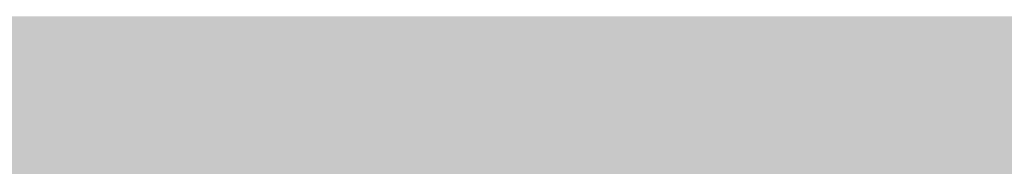
# Model space of a CAD drawing. Units: feet. Extents: x 3168 to 4724, y 827 to 1477.
# Tile 20 of 256: x 3257.497 to 3261.901, y 1098.344 to 1099.001. Entities that reach past the tile are written whole.
import ezdxf

# ---------------------------------------------------------------- set-up
doc = ezdxf.new("R2010")
doc.units = ezdxf.units.FT
doc.layers.add('A-ELEV', color=7, linetype='Continuous', lineweight=35)
doc.layers.add('A-ELEV-PATT', color=8, linetype='Continuous', lineweight=13)

msp = doc.modelspace()

# ---------------------------------------------------------------- hatches: boundary and pattern name
at = {"layer": 'A-ELEV-PATT'}
h = msp.add_hatch(color=256, dxfattribs=at)
h.dxf.hatch_style = 1
edge = h.paths.add_edge_path()
edge.add_ellipse((3552.9058, 979.2201), major_axis=(36.7449, 0), ratio=0.4848485, start_angle=0, end_angle=360)
edge = h.paths.add_edge_path()
edge.add_ellipse((3559.8916, 929.2523), major_axis=(36.7449, 0), ratio=0.4848485, start_angle=0, end_angle=360)
edge = h.paths.add_edge_path()
edge.add_line((3299.3168, 1198.6061), (3479.9167, 1198.6061))
edge.add_line((3479.9167, 1198.6061), (3479.9167, 1209.8686))
edge.add_spline(control_points=[(3479.9167, 1209.8686), (3464.3012, 1209.8686), (3448.6856, 1209.8686), (3410.9491, 1209.8686), (3388.8282, 1209.8686), (3355.6469, 1209.8686), (3344.5864, 1209.8686), (3327.9957, 1209.8686), (3322.4655, 1209.8686), (3314.1702, 1209.8686), (3311.4051, 1209.8686), (3307.2574, 1209.8686), (3305.8748, 1209.8686), (3303.801, 1209.8686), (3303.1097, 1209.8686), (3302.0728, 1209.8686), (3301.7272, 1209.8686), (3301.2087, 1209.8686), (3301.0359, 1209.8686), (3300.7767, 1209.8686), (3300.6903, 1209.8686), (3300.5606, 1209.8686), (3300.5174, 1209.8686), (3300.4526, 1209.8686), (3300.431, 1209.8686), (3300.3986, 1209.8686), (3300.3878, 1209.8686), (3300.3662, 1209.8686), (3300.3457, 1209.8686), (3300.3455, 1209.8686), (3300.3455, 1209.8686), (3300.3433, 1209.8686), (3300.3411, 1209.8686), (3300.3379, 1209.8686), (3300.3368, 1209.8686), (3300.3339, 1209.8686), (3300.3321, 1209.8686), (3300.3255, 1209.8686), (3300.3207, 1209.8686), (3300.3109, 1209.8686), (3300.306, 1209.8686), (3300.2905, 1209.8686), (3300.28, 1209.8686), (3300.2324, 1209.8688), (3300.1953, 1209.869), (3299.9511, 1209.8706), (3299.7448, 1209.8743), (3299.4368, 1209.8833), (3299.3344, 1209.8868), (3299.1811, 1209.8929), (3299.13, 1209.8951), (3298.6522, 1209.9168), (3298.2295, 1209.9457), (3297.6016, 1210.0024), (3297.3934, 1210.0235), (3297.0827, 1210.0583), (3296.9793, 1210.0705), (3296.293, 1210.1549), (3295.7181, 1210.2434), (3294.8687, 1210.3989), (3294.5877, 1210.4545), (3294.1693, 1210.5433), (3294.0304, 1210.5739), (3291.7071, 1211.1012), (3289.6536, 1211.8134), (3285.7763, 1213.564), (3283.9514, 1214.6035), (3280.5122, 1216.9801), (3278.8972, 1218.3176), (3276.3799, 1220.8295), (3275.416, 1221.9177), (3274.0393, 1223.7077), (3273.581, 1224.3495), (3273.1432, 1225.0163)], knot_values=[39.119033, 39.119033, 39.119033, 39.119033, 39.286353, 39.286353, 39.523379, 39.523379, 39.641892, 39.641892, 39.701148, 39.701148, 39.730777, 39.730777, 39.745591, 39.745591, 39.752998, 39.752998, 39.756701, 39.756701, 39.758553, 39.758553, 39.759479, 39.759479, 39.759942, 39.759942, 39.760173, 39.760173, 39.760289, 39.760289, 39.760405, 39.760405, 39.760463, 39.760463, 39.763389, 39.763389, 39.764851, 39.764851, 39.767304, 39.767304, 39.773825, 39.773825, 39.78057, 39.78057, 39.79477, 39.79477, 39.845194, 39.845194, 40.126715, 40.126715, 40.267476, 40.267476, 40.337856, 40.337856, 40.927023, 40.927023, 41.221606, 41.221606, 41.368898, 41.368898, 42.202622, 42.202622, 42.619485, 42.619485, 42.827916, 42.827916, 46.118323, 46.118323, 49.408731, 49.408731, 52.699139, 52.699139, 54.927489, 54.927489, 56.104228, 56.104228, 56.104228, 56.104228], weights=[1, 1, 1, 1, 1, 1, 1, 1, 1, 1, 1, 1, 1, 1, 1, 1, 1, 1, 1, 1, 1, 1, 1, 1, 1, 1, 1, 1, 1, 1, 1, 1, 1, 1, 1, 1, 1, 1, 1, 1, 1, 1, 1, 1, 1, 1, 1, 1, 1, 1, 1, 1, 1, 1, 1, 1, 1, 1, 1, 1, 1, 1, 1, 1, 1, 1, 1, 1, 1, 1, 1, 1, 1, 1], degree=3, periodic=0)
edge.add_line((3273.1432, 1225.0163), (3273.1432, 1099.0163))
edge.add_line((3273.1432, 1099.0163), (3299.3168, 1099.0163))
edge.add_line((3299.3168, 1099.0163), (3299.3168, 1198.6061))
edge = h.paths.add_edge_path()
edge.add_line((3304.7584, 1324.1581), (3479.9167, 1324.1581))
edge.add_line((3479.9167, 1324.1581), (3479.9167, 1335.7146))
edge.add_line((3479.9167, 1335.7146), (3269.1616, 1335.7146))
edge.add_spline(control_points=[(3269.1616, 1335.7146), (3264.0242, 1335.7146), (3258.3641, 1328.9582), (3259.2643, 1323.9003)], knot_values=[0, 0, 0, 0, 15.412191, 15.412191, 15.412191, 15.412191], degree=3, periodic=0)
edge.add_line((3259.2643, 1323.9003), (3265.5168, 1288.7691))
edge.add_line((3265.5168, 1288.7691), (3275.2651, 1261.5456))
edge.add_line((3275.2651, 1261.5456), (3304.7584, 1261.5456))
edge.add_line((3304.7584, 1261.5456), (3304.7584, 1324.1581))
h = msp.add_hatch(color=256, dxfattribs=at)
h.dxf.hatch_style = 1
h.paths.add_polyline_path([(3384.5252, 1099.0163), (3335.0292, 1099.0163), (3299.3168, 1099.0163), (3273.1432, 1099.0163), (3217.5654, 1099.0163), (3168.0693, 827.1163), (3335.0292, 827.1163)])

# ---------------------------------------------------------------- linework, layer by layer
at = {"layer": 'A-ELEV'}
msp.add_open_spline([(3808.5202, 1099.0163), (3808.5202, 1141.4132), (3808.5202, 1183.8102), (3808.5202, 1226.6353), (3808.5202, 1227.0636), (3808.5202, 1227.4918), (3811.4919, 1248.9947), (3814.4635, 1270.4975), (3817.4652, 1292.2176), (3817.4952, 1292.4348), (3817.5253, 1292.652), (3817.5728, 1310.1067), (3817.6203, 1327.5615), (3817.6679, 1345.0163), (3817.6679, 1345.458), (3817.6679, 1345.8996), (3817.6679, 1346.456), (3817.6679, 1346.5708), (3817.6679, 1346.7529), (3817.6679, 1346.8201), (3817.6679, 1346.9349), (3817.6679, 1346.9823), (3817.6679, 1347.0386), (3817.6679, 1347.0474), (3817.6679, 1347.0737), (3817.6679, 1347.0593), (3817.6679, 1347.0615), (3817.6679, 1347.0627), (3817.6679, 1347.066), (3817.6679, 1347.0683), (3817.6679, 1347.075), (3817.6679, 1347.0795), (3817.6678, 1347.0929), (3817.6678, 1347.1019), (3817.6678, 1347.1288), (3817.6677, 1347.1467), (3817.6674, 1347.2004), (3817.6672, 1347.2362), (3817.6661, 1347.3434), (3817.665, 1347.4147), (3817.6608, 1347.6281), (3817.6566, 1347.7697), (3817.64, 1348.1925), (3817.6235, 1348.4716), (3817.5591, 1349.3001), (3817.4961, 1349.8406), (3817.2554, 1351.4242), (3817.0263, 1352.4288), (3816.3069, 1354.8889), (3815.7437, 1356.2687), (3814.464, 1358.8192), (3813.7464, 1359.991), (3812.1958, 1362.1723), (3811.3622, 1363.1821), (3809.5888, 1365.069), (3808.6488, 1365.9461), (3806.6543, 1367.5796), (3805.5997, 1368.3362), (3803.3529, 1369.7223), (3802.1605, 1370.3524), (3799.6008, 1371.4536), (3798.2327, 1371.9255), (3795.2801, 1372.6346), (3793.6931, 1372.8721), (3791.8694, 1372.9265), (3791.7409, 1372.9292), (3791.3534, 1372.9341), (3791.0927, 1372.9329), (3790.3041, 1372.9151), (3789.7695, 1372.8842), (3789.2092, 1372.8302), (3789.1906, 1372.8284), (3789.1349, 1372.8229), (3789.0977, 1372.8191), (3789.0484, 1372.814), (3789.0364, 1372.8127), (3789.0003, 1372.8089), (3788.9761, 1372.8063), (3788.9494, 1372.8034), (3788.9468, 1372.8031), (3788.9426, 1372.8027), (3788.941, 1372.8025), (3788.9386, 1372.8022), (3788.9378, 1372.8021), (3788.9354, 1372.8019), (3788.8675, 1372.7944), (3788.7569, 1372.7822), (3788.7015, 1372.7761), (3788.5355, 1372.7579), (3788.4249, 1372.7457), (3788.0929, 1372.7092), (3787.8715, 1372.6848), (3787.2075, 1372.6118), (3786.7648, 1372.5631), (3785.4368, 1372.417), (3784.5515, 1372.3196), (3781.8954, 1372.0274), (3780.1247, 1371.8327), (3774.8126, 1371.2483), (3771.2713, 1370.8587), (3760.6471, 1369.69), (3753.5643, 1368.9109), (3732.316, 1366.5735), (3718.1504, 1365.0152), (3694.0068, 1362.3593), (3684.0287, 1361.2617), (3674.0506, 1360.1641), (3664.6007, 1360.1641), (3655.1508, 1360.1641), (3626.8011, 1360.1641), (3607.9013, 1360.1641), (3551.2019, 1360.1641), (3513.4023, 1360.1641), (3467.7252, 1360.1641), (3459.8476, 1360.1641), (3436.2149, 1360.1641), (3420.4597, 1360.1641), (3373.1943, 1360.1641), (3341.6839, 1360.1641), (3302.8482, 1360.1641), (3295.5227, 1360.1641), (3286.0383, 1360.1641), (3283.8794, 1360.1641), (3277.4026, 1360.1641), (3273.0848, 1360.1641), (3267.7329, 1360.1641), (3266.6988, 1360.1641), (3263.5965, 1360.1641), (3261.5284, 1360.1641), (3259.2369, 1360.1641), (3259.0137, 1360.1641), (3258.344, 1360.1641), (3257.8975, 1360.1641), (3257.431, 1360.1641), (3257.411, 1360.1641), (3257.3706, 1360.1641), (3257.3755, 1360.1641), (3257.3746, 1360.1641), (3257.3739, 1360.1641), (3257.372, 1360.1641), (3257.3706, 1360.1641), (3257.3667, 1360.1641), (3257.364, 1360.1641), (3257.3561, 1360.1641), (3257.3508, 1360.164), (3257.335, 1360.164), (3257.3244, 1360.164), (3257.2928, 1360.1639), (3257.2717, 1360.1638), (3257.2084, 1360.1634), (3257.1663, 1360.163), (3257.0402, 1360.1614), (3256.9563, 1360.1598), (3256.7055, 1360.1534), (3256.5392, 1360.147), (3256.0436, 1360.1219), (3255.7173, 1360.0971), (3254.7524, 1360.0005), (3254.128, 1359.9065), (3252.1801, 1359.5253), (3250.9416, 1359.144), (3248.6702, 1358.2433), (3247.6357, 1357.7238), (3245.7326, 1356.6035), (3244.8634, 1356.0021), (3243.2531, 1354.7429), (3242.512, 1354.0847), (3240.7511, 1352.3448), (3239.801, 1351.2296), (3238.0878, 1348.8724), (3237.3247, 1347.6304), (3235.9825, 1344.9716), (3235.4022, 1343.5549), (3234.5911, 1340.8155), (3234.3109, 1339.5435), (3233.9765, 1336.8026), (3233.9221, 1335.3309), (3234.1489, 1332.5913), (3234.3495, 1331.3672), (3234.7199, 1329.9994), (3234.7524, 1329.8834), (3234.8536, 1329.5348), (3234.9259, 1329.3017), (3235.0248, 1329.0026), (3235.0469, 1328.9369), (3235.0776, 1328.8472), (3235.0859, 1328.8232), (3235.1109, 1328.7511), (3235.1278, 1328.703), (3235.148, 1328.6462), (3235.1511, 1328.6376), (3235.1561, 1328.6235), (3235.1581, 1328.618), (3235.1602, 1328.612), (3235.1656, 1328.5969), (3235.1801, 1328.5565), (3235.1903, 1328.5281), (3235.2208, 1328.4429), (3235.2411, 1328.3862), (3235.3021, 1328.2159), (3235.3427, 1328.1023), (3235.4647, 1327.7617), (3235.546, 1327.5346), (3235.79, 1326.8534), (3235.9526, 1326.3992), (3236.4405, 1325.0367), (3236.7657, 1324.1284), (3237.7415, 1321.4034), (3238.392, 1319.5868), (3240.3435, 1314.1369), (3241.6445, 1310.5036), (3245.5476, 1299.6037), (3248.1496, 1292.3371), (3255.9557, 1270.5374), (3261.1598, 1256.0042), (3267.3876, 1238.612), (3268.4114, 1235.7529), (3269.5104, 1232.6839), (3269.5856, 1232.4739), (3269.7066, 1232.1359), (3269.7524, 1232.0079), (3269.8273, 1231.7987), (3269.8564, 1231.7176), (3269.9063, 1231.5781), (3269.9272, 1231.5198), (3269.9725, 1231.3934), (3269.9968, 1231.3254), (3270.0265, 1231.2425), (3270.0318, 1231.2277), (3270.0403, 1231.204), (3270.0392, 1231.207), (3270.0394, 1231.2066), (3270.0394, 1231.2064), (3270.0396, 1231.2058), (3270.0398, 1231.2055), (3270.0402, 1231.2043), (3270.0404, 1231.2036), (3270.0413, 1231.2013), (3270.0418, 1231.1998), (3270.0434, 1231.1953), (3270.0445, 1231.1922), (3270.0478, 1231.1832), (3270.0499, 1231.1771), (3270.0564, 1231.159), (3270.0608, 1231.147), (3270.0739, 1231.1108), (3270.0826, 1231.0867), (3270.1089, 1231.0144), (3270.1266, 1230.9663), (3270.1799, 1230.8225), (3270.2159, 1230.7269), (3270.3253, 1230.4415), (3270.4, 1230.2528), (3270.6292, 1229.6914), (3270.7889, 1229.3235), (3271.2865, 1228.2383), (3271.6431, 1227.5398), (3272.7759, 1225.5153), (3273.6142, 1224.2605), (3275.416, 1221.9177), (3276.3799, 1220.8295), (3278.8972, 1218.3176), (3280.5122, 1216.9801), (3283.9514, 1214.6035), (3285.7763, 1213.564), (3289.6536, 1211.8134), (3291.7071, 1211.1012), (3294.0304, 1210.5739), (3294.1693, 1210.5433), (3294.5877, 1210.4545), (3294.8687, 1210.3989), (3295.7181, 1210.2434), (3296.293, 1210.1549), (3296.9793, 1210.0705), (3297.0827, 1210.0583), (3297.3934, 1210.0235), (3297.6016, 1210.0024), (3298.2295, 1209.9457), (3298.6522, 1209.9168), (3299.13, 1209.8951), (3299.1811, 1209.8929), (3299.3344, 1209.8868), (3299.4368, 1209.8833), (3299.7448, 1209.8743), (3299.9511, 1209.8706), (3300.1953, 1209.869), (3300.2324, 1209.8688), (3300.28, 1209.8686), (3300.2905, 1209.8686), (3300.306, 1209.8686), (3300.3109, 1209.8686), (3300.3207, 1209.8686), (3300.3255, 1209.8686), (3300.3321, 1209.8686), (3300.3339, 1209.8686), (3300.3368, 1209.8686), (3300.3379, 1209.8686), (3300.3411, 1209.8686), (3300.3433, 1209.8686), (3300.3455, 1209.8686), (3300.3455, 1209.8686), (3300.3457, 1209.8686), (3300.3662, 1209.8686), (3300.3878, 1209.8686), (3300.3986, 1209.8686), (3300.431, 1209.8686), (3300.4526, 1209.8686), (3300.5174, 1209.8686), (3300.5606, 1209.8686), (3300.6903, 1209.8686), (3300.7767, 1209.8686), (3301.0359, 1209.8686), (3301.2087, 1209.8686), (3301.7272, 1209.8686), (3302.0728, 1209.8686), (3303.1097, 1209.8686), (3303.801, 1209.8686), (3305.8748, 1209.8686), (3307.2574, 1209.8686), (3311.4051, 1209.8686), (3314.1702, 1209.8686), (3322.4655, 1209.8686), (3327.9957, 1209.8686), (3344.5864, 1209.8686), (3355.6469, 1209.8686), (3388.8282, 1209.8686), (3410.9491, 1209.8686), (3477.3119, 1209.8686), (3521.5537, 1209.8686), (3566.8362, 1209.8686), (3567.8769, 1209.8686), (3570.999, 1209.8686), (3573.0804, 1209.8686), (3575.7814, 1209.8686), (3576.4009, 1209.8686), (3577.2958, 1209.8686), (3577.5712, 1209.8686), (3578.3971, 1209.8686), (3578.9478, 1209.8686), (3579.7565, 1209.8686), (3580.0145, 1209.8686), (3580.3427, 1209.8686), (3580.3269, 1209.8686), (3580.3272, 1209.8686), (3580.3273, 1209.8686), (3580.3278, 1209.8686), (3580.3281, 1209.8686), (3580.329, 1209.8686), (3580.3296, 1209.8686), (3580.3314, 1209.8686), (3580.3327, 1209.8686), (3580.3363, 1209.8686), (3580.3388, 1209.8686), (3580.3461, 1209.8686), (3580.351, 1209.8686), (3580.3657, 1209.8685), (3580.3754, 1209.8685), (3580.4048, 1209.8684), (3580.4244, 1209.8684), (3580.4832, 1209.8681), (3580.5224, 1209.8678), (3580.6404, 1209.8666), (3580.7192, 1209.8655), (3580.9563, 1209.8608), (3581.1152, 1209.8561), (3581.5942, 1209.8372), (3581.9164, 1209.8183), (3582.8899, 1209.7424), (3583.548, 1209.6662), (3585.5318, 1209.3606), (3586.8672, 1209.0539), (3589.4715, 1208.2525), (3590.7402, 1207.7579), (3591.9955, 1207.1588), (3592.0578, 1207.1287), (3592.2442, 1207.038), (3592.3677, 1206.9766), (3592.7353, 1206.7904), (3592.9768, 1206.6631), (3593.2445, 1206.5164), (3593.2747, 1206.4998), (3593.3651, 1206.4498), (3593.4251, 1206.4163), (3593.6043, 1206.3153), (3593.7227, 1206.2472), (3593.8572, 1206.1684), (3593.8744, 1206.1583), (3593.9257, 1206.128), (3593.9599, 1206.1078), (3594.0621, 1206.0469), (3594.1298, 1206.0061), (3594.2084, 1205.9582), (3594.2197, 1205.9513), (3594.2534, 1205.9307), (3594.2758, 1205.9169), (3594.343, 1205.8755), (3594.3876, 1205.8479), (3594.4336, 1205.819), (3594.4353, 1205.818), (3594.4402, 1205.8149), (3594.4435, 1205.8129), (3594.4471, 1205.8106), (3594.4475, 1205.8103), (3594.4487, 1205.8096), (3594.4495, 1205.8091), (3594.4504, 1205.8086), (3594.4505, 1205.8085), (3594.4506, 1205.8084), (3594.4674, 1205.7979), (3594.4933, 1205.7817), (3594.5062, 1205.7736), (3594.545, 1205.7492), (3594.5709, 1205.733), (3594.6485, 1205.6844), (3594.7002, 1205.652), (3594.8554, 1205.5547), (3594.9589, 1205.4898), (3595.2694, 1205.2953), (3595.4763, 1205.1656), (3596.0972, 1204.7765), (3596.5111, 1204.5171), (3597.7528, 1203.7388), (3598.5807, 1203.22), (3601.0642, 1201.6636), (3602.7198, 1200.6259), (3607.6868, 1197.513), (3610.9981, 1195.4377), (3620.932, 1189.2119), (3627.5546, 1185.0614), (3647.4225, 1172.6097), (3660.6678, 1164.3086), (3700.4035, 1139.4053), (3726.894, 1122.8031), (3757.2057, 1103.8061), (3761.027, 1101.4112), (3764.8482, 1099.0163), (3745.3283, 1099.0163), (3725.8083, 1099.0163), (3706.2884, 1099.0163), (3706.2884, 1108.4532), (3706.2884, 1117.8902), (3706.2884, 1127.3271), (3710.7508, 1127.3271), (3715.2131, 1127.3271), (3719.6755, 1127.3271)], degree=3, knots=[0, 0, 0, 0, 0.982037, 0.982037, 0.991957, 0.991957, 0.991957, 1.966522, 1.966522, 1.976367, 1.976367, 1.976367, 2.976367, 2.976367, 2.976367, 3.00169, 3.00169, 3.008272, 3.008272, 3.012129, 3.012129, 3.014851, 3.014851, 3.015353, 3.015353, 3.016359, 3.016359, 3.017365, 3.017365, 3.019376, 3.019376, 3.023398, 3.023398, 3.031442, 3.031442, 3.047531, 3.047531, 3.079708, 3.079708, 3.144063, 3.144063, 3.272772, 3.272772, 3.53019, 3.53019, 4.045026, 4.045026, 5.074698, 5.074698, 6.700878, 6.700878, 8.327058, 8.327058, 9.953238, 9.953238, 11.579418, 11.579418, 13.205598, 13.205598, 14.831778, 14.831778, 16.457958, 16.457958, 18.084138, 18.084138, 18.206872, 18.206872, 18.45234, 18.45234, 18.943275, 18.943275, 18.960093, 18.960093, 18.993729, 18.993729, 19.00461, 19.00461, 19.026374, 19.026374, 19.028737, 19.028737, 19.03018, 19.03018, 19.030897, 19.030897, 19.032332, 19.032332, 19.033766, 19.033766, 19.036636, 19.036636, 19.042374, 19.042374, 19.053851, 19.053851, 19.076805, 19.076805, 19.122714, 19.122714, 19.21453, 19.21453, 19.398163, 19.398163, 19.765429, 19.765429, 20.024128, 20.024128, 20.024128, 20.092031, 20.092031, 20.227836, 20.227836, 20.499446, 20.499446, 20.556051, 20.556051, 20.66926, 20.66926, 20.895678, 20.895678, 20.948316, 20.948316, 20.963829, 20.963829, 20.994855, 20.994855, 21.002285, 21.002285, 21.017146, 21.017146, 21.01875, 21.01875, 21.021959, 21.021959, 21.022102, 21.022102, 21.022249, 21.022249, 21.022708, 21.022708, 21.023627, 21.023627, 21.025464, 21.025464, 21.029138, 21.029138, 21.036486, 21.036486, 21.051183, 21.051183, 21.080575, 21.080575, 21.139361, 21.139361, 21.256932, 21.256932, 21.492073, 21.492073, 21.962356, 21.962356, 23.01002, 23.01002, 24.057684, 24.057684, 25.105348, 25.105348, 26.153011, 26.153011, 27.776787, 27.776787, 29.400562, 29.400562, 31.024337, 31.024337, 32.278801, 32.278801, 33.533265, 33.533265, 34.467568, 34.467568, 34.553971, 34.553971, 34.726776, 34.726776, 34.775309, 34.775309, 34.793079, 34.793079, 34.82862, 34.82862, 34.834979, 34.834979, 34.839039, 34.839039, 34.839411, 34.839411, 34.840285, 34.840285, 34.842034, 34.842034, 34.845531, 34.845531, 34.852525, 34.852525, 34.866512, 34.866512, 34.894488, 34.894488, 34.950439, 34.950439, 35.062342, 35.062342, 35.286147, 35.286147, 35.733758, 35.733758, 35.821815, 35.821815, 35.828283, 35.828283, 35.832225, 35.832225, 35.834724, 35.834724, 35.836521, 35.836521, 35.838617, 35.838617, 35.839073, 35.839073, 35.839345, 35.839345, 35.839617, 35.839617, 35.840161, 35.840161, 35.841249, 35.841249, 35.843425, 35.843425, 35.847778, 35.847778, 35.856482, 35.856482, 35.873891, 35.873891, 35.908709, 35.908709, 35.978345, 35.978345, 36.117617, 36.117617, 36.396161, 36.396161, 36.953248, 36.953248, 38.067423, 38.067423, 40.295772, 40.295772, 42.524122, 42.524122, 45.81453, 45.81453, 49.104937, 49.104937, 52.395345, 52.395345, 52.603776, 52.603776, 53.020639, 53.020639, 53.854363, 53.854363, 54.001655, 54.001655, 54.296238, 54.296238, 54.885405, 54.885405, 54.955785, 54.955785, 55.096546, 55.096546, 55.378067, 55.378067, 55.42849, 55.42849, 55.442691, 55.442691, 55.449436, 55.449436, 55.455957, 55.455957, 55.458409, 55.458409, 55.459872, 55.459872, 55.462798, 55.462798, 55.462856, 55.462856, 55.462972, 55.462972, 55.463088, 55.463088, 55.463319, 55.463319, 55.463782, 55.463782, 55.464708, 55.464708, 55.46656, 55.46656, 55.470263, 55.470263, 55.47767, 55.47767, 55.492484, 55.492484, 55.522112, 55.522112, 55.581369, 55.581369, 55.699882, 55.699882, 55.936907, 55.936907, 56.410959, 56.410959, 56.42211, 56.42211, 56.444413, 56.444413, 56.451051, 56.451051, 56.454001, 56.454001, 56.459901, 56.459901, 56.462666, 56.462666, 56.463418, 56.463418, 56.464171, 56.464171, 56.465675, 56.465675, 56.468684, 56.468684, 56.474702, 56.474702, 56.486738, 56.486738, 56.51081, 56.51081, 56.558955, 56.558955, 56.655243, 56.655243, 56.847821, 56.847821, 57.232975, 57.232975, 58.003284, 58.003284, 59.543901, 59.543901, 62.625137, 62.625137, 68.787607, 68.787607, 74.950078, 74.950078, 75.27336, 75.27336, 75.919923, 75.919923, 77.213051, 77.213051, 77.377769, 77.377769, 77.707206, 77.707206, 78.366079, 78.366079, 78.462532, 78.462532, 78.655436, 78.655436, 79.041245, 79.041245, 79.105735, 79.105735, 79.234714, 79.234714, 79.492672, 79.492672, 79.502197, 79.502197, 79.521249, 79.521249, 79.523534, 79.523534, 79.528103, 79.528103, 79.528682, 79.528682, 79.528885, 79.528885, 79.529089, 79.529089, 79.529495, 79.529495, 79.530308, 79.530308, 79.531935, 79.531935, 79.535187, 79.535187, 79.541693, 79.541693, 79.554704, 79.554704, 79.580725, 79.580725, 79.632769, 79.632769, 79.736856, 79.736856, 79.94503, 79.94503, 80.361377, 80.361377, 80.421435, 80.421435, 80.421435, 81.421435, 81.421435, 81.421435, 82.421435, 82.421435, 82.421435, 83.421435, 83.421435, 83.421435, 83.421435], dxfattribs=at)

doc.saveas('drawing.dxf')
